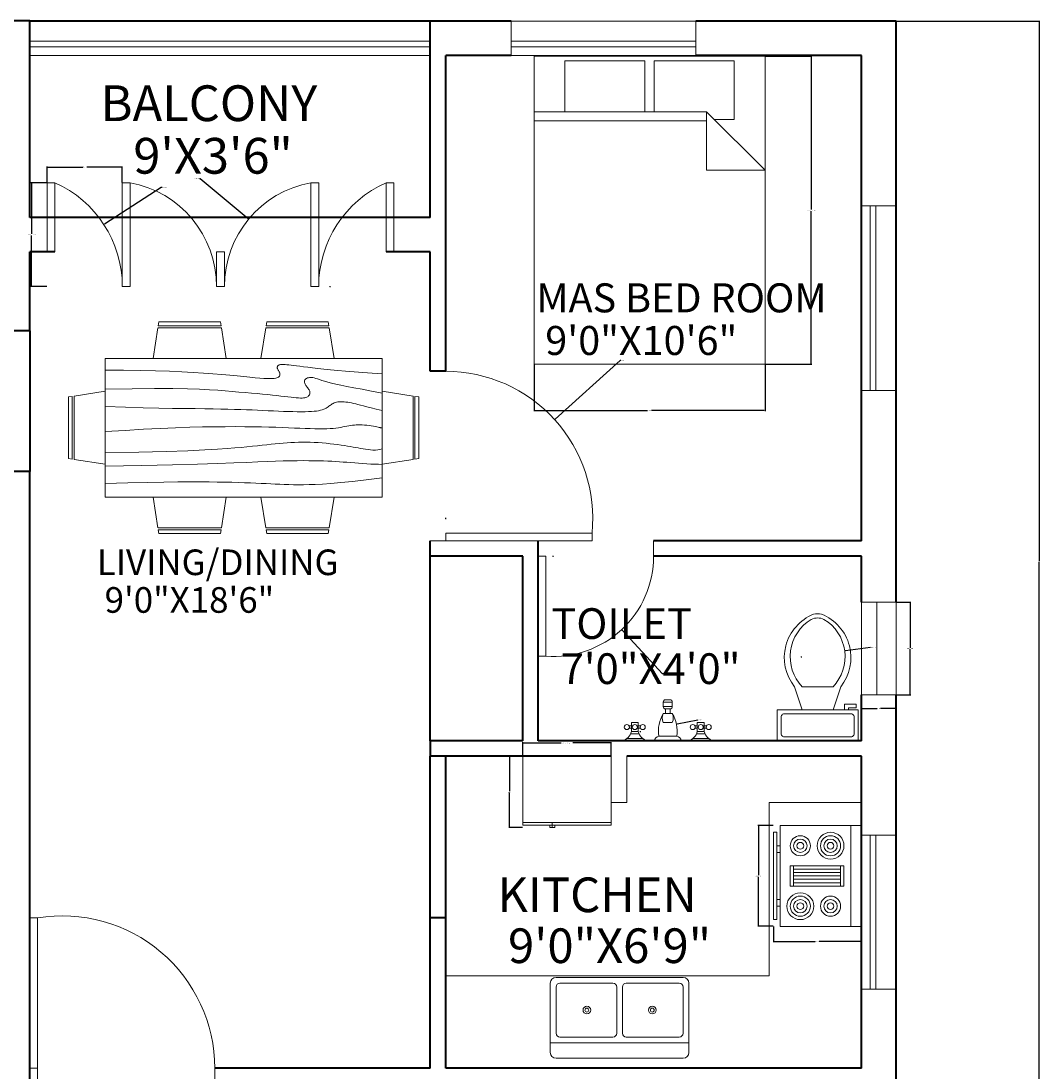
# Model space of a CAD drawing. Units: inches. Extents: x 2220 to 3422, y 783 to 1748.
# Tile 5 of 7: x 2475 to 2740, y 1306 to 1578. Entities that reach past the tile are written whole.
import ezdxf

# ---------------------------------------------------------------- set-up
doc = ezdxf.new("R2010")
doc.units = ezdxf.units.IN
for name, color, linetype, lineweight in [('A-ANNO-DIMS', 2, 'Continuous', 18), ('A-AREA-IDEN', 7, 'Continuous', 18), ('A-DOOR', 3, 'Continuous', 20), ('A-EQPM', 9, 'Continuous', 18), ('A-FLOR-CASE', 8, 'Continuous', 18), ('A-FLOR-FIXT', 9, 'Continuous', 18), ('A-FURN', 8, 'Continuous', 18), ('A-GLAZ', 4, 'Continuous', 18), ('A-WALL', 7, 'Continuous', 40)]:
    doc.layers.add(name, color=color, linetype=linetype, lineweight=lineweight)
doc.styles.get("Standard").update_dxf_attribs({"font": 'arial.ttf'})
doc.dimstyles.get("Standard").update_dxf_attribs({"dimtxt": 0.18, "dimasz": 0.18, "dimexe": 0.18, "dimexo": 0.0625, "dimgap": 0.09, "dimtad": 0, "dimtih": 1, "dimtoh": 1, "dimdec": 4, "dimzin": 0, "dimdsep": 46, "dimtxsty": 'Standard', "dimcen": 0.09, "dimadec": 0, "dimazin": 0, "dimtfac": 1, "dimtdec": 4, "dimtofl": 0, "dimtmove": 0, "dimatfit": 3, "dimfxl": 1, "dimtolj": 1, "dimtzin": 0, "dimarcsym": 0})

# ---------------------------------------------------------------- blocks, each defined once
blk = doc.blocks.new('Range-Oven - 30 in top')
for p, q in [((0, -3), (30, -3)), ((12, -6), (18, -6)), ((13, -20), (13, -6)), ((14, -6), (14, -20)), ((15, -20), (15, -6)), ((16, -6), (16, -20)), ((17, -20), (17, -6)), ((18, -20), (12, -20)), ((6, -24), (6, -25)), ((8, -25), (8, -24)), ((22, -25), (22, -24)), ((24, -24), (24, -25))]:
    blk.add_line(p, q)
for points in [[(0, -24), (0, 0), (30, 0), (30, -24)], [(12, -21), (12, -5), (18, -5), (18, -21)], [(2, -26), (2, -25), (28, -25), (28, -26)]]:
    blk.add_lwpolyline(points, close=True)
for centre, radius in [((6, -9), 4), ((6, -9), 3), ((24, -9), 3), ((6, -9), 2), ((6, -9), 1), ((24, -9), 2), ((24, -9), 1), ((6, -18), 3), ((24, -18), 4), ((24, -18), 3), ((6, -18), 2), ((6, -18), 1), ((24, -18), 2), ((24, -18), 1)]:
    blk.add_circle(centre, radius)
blk = doc.blocks.new('Refrigerator-2 door - 36 in top')
for p, q in [((0, -26.999999), (36, -26.999999)), ((11, -27.999999), (11, -28.999999)), ((11, -28.999999), (13, -28.999999)), ((12, -26.999999), (12, -28.999999)), ((13, -28.999999), (13, -27.999999))]:
    blk.add_line(p, q)
blk.add_lwpolyline([(0, -27.999999), (0, 0), (36, 0), (36, -27.999999)], close=True)
blk = doc.blocks.new('Sink-double - 36 in top')
for p, q in [((-18, -4), (18, -4)), ((-0.75, -18.5), (-0.75, -6.5)), ((0.75, -6.5), (0.75, -18.5))]:
    blk.add_line(p, q)
for points in [[(-16.5, 0), (16.5, 0)], [(-18, -19.5), (-18, -1.5)], [(18, -1.5), (18, -19.5)], [(-16.5, -18.5), (-16.5, -6.5)], [(-15.5, -5.5), (-1.75, -5.5)], [(1.75, -5.5), (15.5, -5.5)], [(16.5, -6.5), (16.5, -18.5)], [(16.5, -21), (-16.5, -21)], [(-1.75, -19.5), (-15.5, -19.5)], [(15.5, -19.5), (1.75, -19.5)]]:
    blk.add_lwpolyline(points)
for centre, radius in [((-8.5, -12.5), 1), ((-8.5, -12.5), 0.5), ((8.5, -12.5), 1), ((8.5, -12.5), 0.5)]:
    blk.add_circle(centre, radius)
for centre, radius, start, end in [((-16.5, -1.5), 1.5, 90, 180), ((16.5, -1.5), 1.5, 0, 90), ((-15.5, -6.5), 1, 90, 180), ((-1.75, -6.5), 1, 0, 90), ((1.75, -6.5), 1, 90, 180), ((15.5, -6.5), 1, 0, 90), ((-15.5, -18.5), 1, 180, 270), ((-1.75, -18.5), 1, 270, 0), ((1.75, -18.5), 1, 180, 270), ((15.5, -18.5), 1, 270, 0), ((-16.5, -19.5), 1.5, 180, 270), ((16.5, -19.5), 1.5, 270, 0)]:
    blk.add_arc(centre, radius, start, end)
blk = doc.blocks.new('Dining Set - 36 x 72 in.')
for p, q in [((-22, 27.5), (-22.1562, 26.50042)), ((-22, 27.5), (-6, 27.5)), ((-5.8437, 26.49966), (-6, 27.5)), ((6, 27.5), (5.8438, 26.50042)), ((6, 27.5), (22, 27.5)), ((22.1563, 26.49966), (22, 27.5)), ((-22.2343, 26.00059), (-23.4847, 17.99762)), ((-22.2304, 26), (-5.7608, 26)), ((-5.8416, 26.5), (-22.1534, 26.5)), ((-4.5152, 17.99762), (-5.7655, 25.99926)), ((5.7657, 26.00059), (4.5153, 17.99762)), ((5.7696, 26), (22.2392, 26)), ((22.1584, 26.5), (5.8466, 26.5)), ((23.4848, 17.99762), (22.2345, 25.99926)), ((36, 18), (-36, 18)), ((-36, 18), (-36, -18)), ((36, -18), (36, 18)), ((-44.0006, 8.23428), (-35.9976, 9.48474)), ((-44, 8.23041), (-44, -8.23915)), ((44.0006, 8.23428), (35.9976, 9.48474)), ((44, 8.23041), (44, -8.23915)), ((-45.5, 8), (-44.5004, 8.15617)), ((-45.5, 8), (-45.5, -8)), ((-44.5, -8.15843), (-44.5, 8.15338)), ((44.5, -8.15843), (44.5, 8.15338)), ((45.5, 8), (44.5005, 8.15617)), ((45.5, 8), (45.5, -8)), ((-44.4997, -8.15631), (-45.5, -8)), ((44.4997, -8.15631), (45.5, -8)), ((-35.9976, -9.48476), (-43.9993, -8.2345)), ((35.9976, -9.48476), (43.9993, -8.2345)), ((-36, -18), (36, -18)), ((-22.2343, -26.0006), (-23.4847, -17.99762)), ((-4.5152, -17.99762), (-5.7655, -25.99928)), ((5.7657, -26.0006), (4.5153, -17.99762)), ((23.4848, -17.99762), (22.2345, -25.99928)), ((-22.2304, -26), (-5.7608, -26)), ((-22, -27.5), (-22.1562, -26.50044)), ((-5.8416, -26.5), (-22.1534, -26.5)), ((-5.8437, -26.49967), (-6, -27.5)), ((5.7696, -26), (22.2392, -26)), ((6, -27.5), (5.8438, -26.50044)), ((22.1584, -26.5), (5.8466, -26.5)), ((22.1563, -26.49967), (22, -27.5)), ((-22, -27.5), (-6, -27.5)), ((6, -27.5), (22, -27.5))]:
    blk.add_line(p, q)
for points in [[(-36, 15), (-31.1772, 14.97754), (-26.8079, 14.91406), (-22.8538, 14.81543), (-19.276, 14.6875), (-16.0362, 14.53613), (-13.0957, 14.36718), (-10.4159, 14.18652), (-7.9583, 14), (-5.6904, 13.81315), (-3.6035, 13.63021), (-1.6954, 13.45508), (0.0365, 13.29166), (1.5945, 13.14388), (2.9811, 13.01562), (4.1988, 12.9108), (5.25, 12.83333), (6.1393, 12.78613), (6.8802, 12.76823), (7.4883, 12.77767), (7.9792, 12.8125), (8.3685, 12.87077), (8.6719, 12.95052), (8.9049, 13.0498), (9.0833, 13.16666), (9.2205, 13.29899), (9.3216, 13.44401), (9.3895, 13.59879), (9.4271, 13.76041), (9.4373, 13.92594), (9.4232, 14.09245), (9.3875, 14.257), (9.3333, 14.41666), (9.2638, 14.56917), (9.1836, 14.71484), (9.0975, 14.85465), (9.0104, 14.98958), (8.9272, 15.1206), (8.8529, 15.2487), (8.7922, 15.37483), (8.75, 15.5), (8.7305, 15.62467), (8.7344, 15.74739), (8.7617, 15.86621), (8.8125, 15.97916), (8.8867, 16.08431), (8.9844, 16.17968), (9.1055, 16.26334), (9.25, 16.33333), (9.4189, 16.38802), (9.6172, 16.42708), (9.8506, 16.45052), (10.125, 16.45833), (10.4463, 16.45052), (10.8203, 16.42708), (11.2529, 16.38802), (11.75, 16.33333), (12.3184, 16.26318), (12.9694, 16.17838), (13.7151, 16.07991), (14.5677, 15.96875), (15.5395, 15.84586), (16.6426, 15.71224), (17.8893, 15.56884), (19.2917, 15.41666), (20.859, 15.25667), (22.5879, 15.08984), (24.4721, 14.91715), (26.5052, 14.73958), (28.6809, 14.5581), (30.9929, 14.3737), (33.4347, 14.18733), (36, 14)], [(-36, 10), (-28.9766, 10.14274), (-23.1725, 10.20442), (-18.4241, 10.19775), (-14.5677, 10.13541), (-11.4399, 10.03011), (-8.877, 9.89453), (-6.7154, 9.74137), (-4.7917, 9.58333), (-2.9698, 9.43082), (-1.2246, 9.28515), (0.4415, 9.14534), (2.026, 9.01041), (3.5266, 8.87939), (4.9408, 8.7513), (6.266, 8.62516), (7.5, 8.5), (8.6411, 8.37549), (9.6914, 8.2539), (10.6538, 8.13818), (11.5312, 8.03125), (12.3267, 7.93603), (13.043, 7.85547), (13.6831, 7.79248), (14.25, 7.75), (14.7471, 7.7303), (15.1797, 7.73307), (15.5537, 7.75732), (15.875, 7.80208), (16.1494, 7.86637), (16.3828, 7.94922), (16.5811, 8.04964), (16.75, 8.16666), (16.8944, 8.29915), (17.0143, 8.44531), (17.1089, 8.60319), (17.1771, 8.77083), (17.218, 8.94629), (17.2305, 9.1276), (17.2137, 9.31282), (17.1667, 9.5), (17.0895, 9.6875), (16.987, 9.875), (16.8649, 10.0625), (16.7292, 10.25), (16.5856, 10.4375), (16.4401, 10.625), (16.2985, 10.8125), (16.1667, 11), (16.05, 11.18733), (15.9518, 11.3737), (15.8752, 11.5581), (15.8229, 11.73958), (15.798, 11.91715), (15.8034, 12.08984), (15.842, 12.25667), (15.9167, 12.41666), (16.0295, 12.56836), (16.1784, 12.70833), (16.3605, 12.83268), (16.5729, 12.9375), (16.8127, 13.01888), (17.0768, 13.07291), (17.3625, 13.0957), (17.6667, 13.08333), (17.9894, 13.03312), (18.3418, 12.94726), (18.7382, 12.82918), (19.1927, 12.68229), (19.7195, 12.51001), (20.3327, 12.31575), (21.0465, 12.10294), (21.875, 11.875), (22.8357, 11.63354), (23.959, 11.37304), (25.2786, 11.08618), (26.8282, 10.76562), (28.6414, 10.40405), (30.752, 9.99414), (33.1936, 9.52856), (36, 9)], [(-36, 5.5), (-30.7157, 5.3348), (-26.069, 5.20963), (-21.9946, 5.11767), (-18.4271, 5.05208), (-15.3009, 5.00602), (-12.5508, 4.97265), (-10.1112, 4.94515), (-7.9167, 4.91666), (-5.909, 4.88167), (-4.0586, 4.83984), (-2.3429, 4.79215), (-0.7396, 4.73958), (0.7739, 4.6831), (2.22, 4.6237), (3.6213, 4.56233), (5, 4.5), (6.373, 4.43782), (7.7344, 4.3776), (9.0723, 4.32129), (10.375, 4.27083), (11.6309, 4.22819), (12.8281, 4.19531), (13.9551, 4.17415), (15, 4.16666), (15.954, 4.17448), (16.819, 4.19791), (17.6001, 4.23698), (18.3021, 4.29166), (18.9299, 4.36198), (19.4883, 4.44791), (19.9823, 4.54948), (20.4167, 4.66666), (20.7969, 4.79899), (21.1302, 4.94401), (21.4245, 5.09879), (21.6875, 5.26041), (21.9271, 5.42594), (22.1511, 5.59245), (22.3672, 5.757), (22.5834, 5.91666), (22.8065, 6.06868), (23.0404, 6.21093), (23.2879, 6.34147), (23.5521, 6.45833), (23.8358, 6.55957), (24.142, 6.64323), (24.4735, 6.70735), (24.8334, 6.75), (25.2235, 6.76969), (25.642, 6.76692), (26.0858, 6.74267), (26.5521, 6.69791), (27.0379, 6.63362), (27.5404, 6.55078), (28.0565, 6.45036), (28.5834, 6.33333), (29.1242, 6.19987), (29.7071, 6.04687), (30.3661, 5.87044), (31.1354, 5.66666), (32.0493, 5.43164), (33.142, 5.16146), (34.4475, 4.85221), (36, 4.5)], [(-36, -1), (-30.7915, -0.6591), (-26.0195, -0.38216), (-21.6519, -0.16284), (-17.6563, 0.00521), (-14.0005, 0.12833), (-10.6523, 0.21289), (-7.5796, 0.26522), (-4.75, 0.29166), (-2.134, 0.29793), (0.2878, 0.28711), (2.5317, 0.26163), (4.6146, 0.22396), (6.5529, 0.17651), (8.3633, 0.12174), (10.0623, 0.06209), (11.6667, 0), (13.1899, -0.06201), (14.6341, -0.1211), (15.9982, -0.17432), (17.2813, -0.21875), (18.4823, -0.25147), (19.6003, -0.26953), (20.6343, -0.27002), (21.5834, -0.25), (22.4481, -0.20768), (23.2357, -0.14584), (23.9549, -0.06836), (24.6146, 0.02083), (25.2235, 0.11784), (25.7904, 0.21875), (26.3241, 0.31966), (26.8334, 0.41666), (27.3265, 0.50618), (27.8099, 0.58593), (28.2894, 0.65397), (28.7709, 0.70833), (29.2601, 0.74707), (29.763, 0.76823), (30.2855, 0.76985), (30.8334, 0.75), (31.4088, 0.70784), (31.9994, 0.64713), (32.589, 0.57275), (33.1615, 0.48958), (33.7008, 0.4025), (34.1908, 0.3164), (34.6153, 0.23616), (34.9584, 0.16666), (35.2099, 0.11165), (35.3848, 0.07031), (35.504, 0.04069), (35.5886, 0.02083), (35.6594, 0.00879), (35.7377, 0.0026), (35.8442, 0.00032), (36, 0)], [(-36, -6.5), (-27.1843, -6.31267), (-20.084, -6.1263), (-14.469, -5.9419), (-10.1094, -5.76042), (-6.7752, -5.58285), (-4.2363, -5.41016), (-2.2629, -5.24333), (-0.625, -5.08334), (0.8708, -4.93099), (2.2715, -4.78646), (3.5872, -4.64974), (4.8281, -4.52084), (6.0046, -4.39974), (7.127, -4.28646), (8.2053, -4.18099), (9.25, -4.08334), (10.2705, -3.99382), (11.2734, -3.91407), (12.2647, -3.84603), (13.25, -3.79167), (14.2354, -3.75293), (15.2266, -3.73177), (16.2295, -3.73015), (17.25, -3.75), (18.2912, -3.79248), (19.3451, -3.85547), (20.4009, -3.93604), (21.4479, -4.03125), (22.4754, -4.13819), (23.4727, -4.25391), (24.4289, -4.37549), (25.3334, -4.5), (26.1785, -4.62492), (26.9694, -4.74935), (27.7145, -4.87281), (28.4219, -4.99479), (29.1, -5.11483), (29.7572, -5.23242), (30.4016, -5.34709), (31.0417, -5.45834), (31.6837, -5.56437), (32.3262, -5.65821), (32.9658, -5.73153), (33.599, -5.77604), (34.2224, -5.78345), (34.8327, -5.74545), (35.4264, -5.65373), (36, -5.5)], [(-36, -10), (-26.4022, -9.81299), (-18.4675, -9.62891), (-11.9839, -9.45069), (-6.7396, -9.28125), (-2.5226, -9.12354), (0.8789, -8.98047), (3.6769, -8.85498), (6.0833, -8.75), (8.2767, -8.66765), (10.3021, -8.60677), (12.1712, -8.56543), (13.8958, -8.54167), (15.4876, -8.53353), (16.9583, -8.53907), (18.3197, -8.55632), (19.5834, -8.58334), (20.7616, -8.61841), (21.8685, -8.66081), (22.9188, -8.71004), (23.9271, -8.76563), (24.9081, -8.82707), (25.8763, -8.89388), (26.8465, -8.96558), (27.8334, -9.04167), (28.8474, -9.12118), (29.8828, -9.20117), (30.93, -9.27824), (31.9792, -9.34896), (33.0205, -9.40991), (34.0443, -9.45768), (35.0407, -9.48885), (36, -9.5)], [(-36, -14.5), (-30.0881, -14.33513), (-25.0332, -14.21224), (-20.7312, -14.12647), (-17.0781, -14.07292), (-13.97, -14.04671), (-11.3027, -14.04297), (-8.9724, -14.05681), (-6.875, -14.08334), (-4.9224, -14.11833), (-3.0905, -14.16016), (-1.3709, -14.20785), (0.2448, -14.26042), (1.7647, -14.3169), (3.1973, -14.3763), (4.5507, -14.43767), (5.8333, -14.5), (7.0554, -14.5621), (8.235, -14.62175), (9.3922, -14.67652), (10.5469, -14.72396), (11.7192, -14.76164), (12.929, -14.78711), (14.1965, -14.79794), (15.5417, -14.79167), (16.9933, -14.76424), (18.6152, -14.70508), (20.4804, -14.60197), (22.6615, -14.44271), (25.2312, -14.21509), (28.2624, -13.9069), (31.8277, -13.50594), (36, -13)]]:
    blk.add_lwpolyline(points)
blk = doc.blocks.new('Toilet - top')
for p, q in [((9.5, -6), (9.5, -2)), ((-8, -8.5), (-8, -8)), ((-7, -8), (-7, -9.5)), ((-4, -8), (-6, -14)), ((4, -8), (6, -14)), ((-10, -8.5), (-8, -8.5)), ((-10, -9.5), (-10, -8.5)), ((-7, -9.5), (-10, -9.5)), ((4, -14), (-4, -14))]:
    blk.add_line(p, q)
blk.add_lwpolyline([(10.5, -8), (10.5, 0), (-10.5, 0), (-10.5, -8)], close=True)
for points in [[(-9.5, -2), (-9.5, -6)], [(8.5, -1), (-8.5, -1)], [(-8.5, -7), (8.5, -7)]]:
    blk.add_lwpolyline(points)
for centre, radius, start, end in [((-8.62, -1.88), 0.884, 81.8699, 188.1301), ((8.62, -1.88), 0.884, 351.8699, 98.1301), ((-8.62, -6.12), 0.884, 171.8699, 278.1301), ((8.62, -6.12), 0.884, 261.8699, 8.1301), ((3.52, -21.58), 12.17, 141.4691, 247.9714), ((4.2, -21.82), 11.33, 136.3677, 238.9468), ((-3.52, -21.58), 12.17, 292.0284, 38.5307), ((-4.2, -21.82), 11.33, 301.053, 43.6321), ((0, -27.88), 4, 245.7318, 294.2682), ((0, -29), 4, 254.8605, 285.1395)]:
    blk.add_arc(centre, radius, start, end)
blk = doc.blocks.new('Faucet - Bathroom front')
for p, q in [((-0.5, 4.25), (0.5, 4.25)), ((0.5, 3.75), (-0.5, 3.75)), ((-0.25, 3), (-0.25, 3.5)), ((0.25, 3.5), (0.25, 3)), ((-0.5, 3), (0.5, 3)), ((-4, 1.625), (-4.25, 1.625)), ((-4, 1.375), (-4.25, 1.375)), ((-3.25, 1.625), (-3, 1.625)), ((-3.25, 1.375), (-3, 1.375)), ((0.5, 2), (-0.5, 2)), ((3.25, 1.625), (3, 1.625)), ((3.25, 1.375), (3, 1.375)), ((4, 1.625), (4.25, 1.625)), ((4, 1.375), (4.25, 1.375)), ((-5, 0), (-2.25, 0)), ((-4.5087, 0.25), (-2.7408, 0.25)), ((-3.1442, 0.75), (-4.0979, 0.75)), ((-1.5, 0), (1.5, 0)), ((-1, 0.5), (1, 0.5)), ((2.25, 0), (5, 0)), ((2.7413, 0.25), (4.5092, 0.25)), ((4.1058, 0.75), (3.1521, 0.75))]:
    blk.add_line(p, q)
for points in [[(-0.5, 3.75), (-0.5, 4.25)], [(-0.25, 4.5), (0.25, 4.5)], [(0.25, 3.5), (-0.25, 3.5)], [(0.5, 4.25), (0.5, 3.75)]]:
    blk.add_lwpolyline(points)
for points in [[(-4, 1), (-4, 2), (-3.25, 2), (-3.25, 1)], [(3.25, 1), (3.25, 2), (4, 2), (4, 1)]]:
    blk.add_lwpolyline(points, close=True)
for centre in [(-4.5, 1.5), (-3.625, 1.5), (-2.75, 1.5), (2.75, 1.5), (3.625, 1.5), (4.5, 1.5)]:
    blk.add_circle(centre, 0.2795)
for centre, radius, start, end in [((-0.2575, 4.2575), 0.2426, 88.22243, 181.7776), ((-0.2575, 3.7425), 0.2426, 178.2224, 271.7776), ((0.2575, 4.2575), 0.2426, 358.2224, 91.77757), ((0.2575, 3.7425), 0.2426, 268.2224, 1.777565), ((3, 1), 4.0311, 150.2551, 187.125), ((0.6413, 2.5), 1.246, 156.3417, 203.6583), ((-3, 1), 4.0311, 352.875, 29.74488), ((-0.6413, 2.5), 1.246, 336.3417, 23.65835), ((-5.375, 1.375), 1.4252, 285.2551, 344.7449), ((-1.875, 1.375), 1.4252, 195.2551, 254.7449), ((-0.7962, -0.2038), 0.7327, 106.1502, 163.8498), ((0.7962, -0.2038), 0.7327, 16.1502, 73.84979), ((1.875, 1.375), 1.4252, 285.2551, 344.7449), ((5.375, 1.375), 1.4252, 195.2551, 254.7449)]:
    blk.add_arc(centre, radius, start, end)
blk = doc.blocks.new('Bed - Queen')
for p, q in [((0, -80.00003), (0, 0)), ((0, 0), (59.99999, 0)), ((59.99999, 0), (59.99999, -80.00003)), ((7.99999, -1.2), (28.79998, -1.2)), ((7.99999, -14.4), (7.99999, -1.2)), ((28.79998, -1.2), (28.79998, -14.4)), ((31.19999, -1.2), (51.99999, -1.2)), ((31.19999, -14.4), (31.19999, -1.2)), ((51.99999, -1.2), (51.99999, -16.4)), ((0, -14.4), (44.8, -14.4)), ((59.99999, -29.6), (44.8, -14.4)), ((44.8, -14.4), (44.8, -29.6)), ((44.8, -16.8), (0, -16.8)), ((51.99999, -16.4), (46.79936, -16.4)), ((44.8, -29.6), (59.99999, -29.6)), ((59.99999, -80.00003), (0, -80.00003))]:
    blk.add_line(p, q)
blk = doc.blocks.new('DOOR-UNIT-ENTRY')
for p, q in [((0, 48.53), (2, 48.53)), ((2, 0.53), (2, 48.53)), ((48, 39.53), (48, 48.53)), ((0, 39.53), (2, 39.53)), ((0, 0.53), (2, 0.53))]:
    blk.add_line(p, q)
blk.add_arc((8.47, 39.53), 39.53, 260.5843, 0)
blk = doc.blocks.new('DOOR-BATH-SWING')
for p, q in [((30, 26.06), (30, 30.06)), ((0, 26.06), (2, 26.06)), ((2, 0.06), (2, 26.06)), ((0, 0.06), (2, 0.06))]:
    blk.add_line(p, q)
blk.add_arc((3.93, 26.06), 26.07, 265.7578, 0)
blk = doc.blocks.new('DOOR-BALCONY-CENTER')
for p, q in [((0, 0), (0, 27)), ((0, 27), (2, 27)), ((2, 0), (2, 27)), ((24.5, 27), (24.5, 18)), ((24.5, 27), (26.5, 27)), ((26.5, 27), (26.5, 18)), ((49, 27), (49, 0)), ((49, 27), (51, 27)), ((51, 27), (51, 0)), ((0, 0), (2, 0)), ((49, 0), (51, 0))]:
    blk.add_line(p, q)
for centre, start, end in [((-2.95, 27), 280.3889, 0), ((53.95, 27), 180, 259.6111)]:
    blk.add_arc(centre, 27.45, start, end)
blk = doc.blocks.new('DOOR-BALCONY-END-B')
for p, q in [((0, 27), (0, 9)), ((0, 27), (2, 27)), ((2, 27), (2, 9))]:
    blk.add_line(p, q)
blk.add_arc((-10.08, 0), 29.58, 0, 65.8984)
blk = doc.blocks.new('WIN-48-OFFSET-A')
for p, q in [((0, 0), (0, 9)), ((0, 9), (48, 9)), ((48, 0), (48, 9)), ((0, 6.75), (48, 6.75)), ((0, 5.25), (48, 5.25)), ((0, 0), (48, 0))]:
    blk.add_line(p, q)
blk = doc.blocks.new('VENT-24-SINGLE')
for p, q in [((0, 24), (9, 24)), ((0, 24), (0, 0)), ((4, 0), (4, 24)), ((9, 24), (9, 0)), ((0, 0), (9, 0))]:
    blk.add_line(p, q)
blk = doc.blocks.new('*D19')
at = {"layer": 'A-ANNO-DIMS', "color": 0, "lineweight": -2, "transparency": 16777216}
for p, q in [((2668.55, 1569.22), (2680.66, 1569.22)), ((2680.48, 1569.04), (2680.48, 1529.41)), ((2680.48, 1489.4), (2680.48, 1529.03)), ((2668.55, 1489.22), (2680.66, 1489.22))]:
    blk.add_line(p, q, dxfattribs=at)
at = {"layer": 'A-ANNO-DIMS', "color": 0, "transparency": 16777216}
for points in [[(2680.45, 1569.04), (2680.51, 1569.04), (2680.48, 1569.22)], [(2680.45, 1489.4), (2680.51, 1489.4), (2680.48, 1489.22)]]:
    blk.add_solid(points, dxfattribs=at)
at = {"layer": 'Defpoints', "color": 0, "transparency": 16777216}
for p in [(2668.48, 1569.22), (2680.48, 1569.22), (2668.48, 1489.22)]:
    blk.add_point(p, dxfattribs=at)
at = {"layer": 'A-ANNO-DIMS', "color": 0, "transparency": 16777216, "insert": (2680.48, 1529.22), "char_height": 0.18, "attachment_point": 5}
blk.add_mtext('\\A1;QUEEN BED 80 TYP.', dxfattribs=at)
blk = doc.blocks.new('*D20')
at = {"layer": 'A-ANNO-DIMS', "color": 0, "lineweight": -2, "transparency": 16777216}
for p, q in [((2608.48, 1489.16), (2608.48, 1477.04)), ((2668.48, 1489.16), (2668.48, 1477.04)), ((2608.66, 1477.22), (2637.95, 1477.22)), ((2668.3, 1477.22), (2639.01, 1477.22))]:
    blk.add_line(p, q, dxfattribs=at)
at = {"layer": 'A-ANNO-DIMS', "color": 0, "transparency": 16777216}
for points in [[(2608.66, 1477.25), (2608.66, 1477.19), (2608.48, 1477.22)], [(2668.3, 1477.25), (2668.3, 1477.19), (2668.48, 1477.22)]]:
    blk.add_solid(points, dxfattribs=at)
at = {"layer": 'Defpoints', "color": 0, "transparency": 16777216}
for p in [(2608.48, 1489.22), (2668.48, 1489.22), (2668.48, 1477.22)]:
    blk.add_point(p, dxfattribs=at)
at = {"layer": 'A-ANNO-DIMS', "color": 0, "transparency": 16777216, "insert": (2638.48, 1477.22), "char_height": 0.18, "attachment_point": 5}
blk.add_mtext('\\A1;60 TYP.', dxfattribs=at)
blk = doc.blocks.new('*D27')
at = {"layer": 'A-ANNO-DIMS', "color": 0, "lineweight": -2, "transparency": 16777216}
for p, q in [((2670.61, 1369.38), (2666.57, 1369.38)), ((2666.75, 1369.2), (2666.75, 1356.48)), ((2666.75, 1343.4), (2666.75, 1356.12)), ((2670.61, 1343.22), (2666.57, 1343.22))]:
    blk.add_line(p, q, dxfattribs=at)
at = {"layer": 'A-ANNO-DIMS', "color": 0, "transparency": 16777216}
for points in [[(2666.72, 1369.2), (2666.78, 1369.2), (2666.75, 1369.38)], [(2666.72, 1343.4), (2666.78, 1343.4), (2666.75, 1343.22)]]:
    blk.add_solid(points, dxfattribs=at)
at = {"layer": 'Defpoints', "color": 0, "transparency": 16777216}
for p in [(2670.68, 1369.38), (2666.75, 1343.22), (2670.68, 1343.22)]:
    blk.add_point(p, dxfattribs=at)
at = {"layer": 'A-ANNO-DIMS', "color": 0, "transparency": 16777216, "insert": (2666.75, 1356.3), "char_height": 0.18, "attachment_point": 5}
blk.add_mtext('\\A1;RANGE 26 TYP.', dxfattribs=at)
blk = doc.blocks.new('*D28')
at = {"layer": 'A-ANNO-DIMS', "color": 0, "lineweight": -2, "transparency": 16777216}
for p, q in [((2670.68, 1343.16), (2670.68, 1339.11)), ((2693.35, 1343.16), (2693.35, 1339.11)), ((2670.86, 1339.29), (2681.48, 1339.29)), ((2693.17, 1339.29), (2682.54, 1339.29))]:
    blk.add_line(p, q, dxfattribs=at)
at = {"layer": 'A-ANNO-DIMS', "color": 0, "transparency": 16777216}
for points in [[(2670.86, 1339.32), (2670.86, 1339.26), (2670.68, 1339.29)], [(2693.17, 1339.32), (2693.17, 1339.26), (2693.35, 1339.29)]]:
    blk.add_solid(points, dxfattribs=at)
at = {"layer": 'Defpoints', "color": 0, "transparency": 16777216}
for p in [(2670.68, 1343.22), (2693.35, 1343.22), (2693.35, 1339.29)]:
    blk.add_point(p, dxfattribs=at)
at = {"layer": 'A-ANNO-DIMS', "color": 0, "transparency": 16777216, "insert": (2682.01, 1339.29), "char_height": 0.18, "attachment_point": 5}
blk.add_mtext('\\A1;23 TYP.', dxfattribs=at)
blk = doc.blocks.new('*D37')
at = {"layer": 'A-ANNO-DIMS', "color": 0, "lineweight": -2, "transparency": 16777216}
for p, q in [((2605.54, 1387.48), (2605.54, 1391.05)), ((2628.55, 1387.48), (2628.55, 1391.05)), ((2605.72, 1390.87), (2615.49, 1390.87)), ((2628.37, 1390.87), (2618.6, 1390.87))]:
    blk.add_line(p, q, dxfattribs=at)
at = {"layer": 'A-ANNO-DIMS', "color": 0, "transparency": 16777216}
for points in [[(2605.72, 1390.9), (2605.72, 1390.84), (2605.54, 1390.87)], [(2628.37, 1390.9), (2628.37, 1390.84), (2628.55, 1390.87)]]:
    blk.add_solid(points, dxfattribs=at)
at = {"layer": 'Defpoints', "color": 0, "transparency": 16777216}
for p in [(2628.55, 1390.87), (2605.54, 1387.41), (2628.55, 1387.41)]:
    blk.add_point(p, dxfattribs=at)
at = {"layer": 'A-ANNO-DIMS', "color": 0, "transparency": 16777216, "insert": (2617.04, 1390.87), "char_height": 0.18, "attachment_point": 5}
blk.add_mtext('\\A1;REFRIGERATOR 23 TYP.', dxfattribs=at)
blk = doc.blocks.new('*D38')
at = {"layer": 'A-ANNO-DIMS', "color": 0, "lineweight": -2, "transparency": 16777216}
for p, q in [((2605.48, 1387.41), (2601.91, 1387.41)), ((2602.09, 1387.23), (2602.09, 1378.33)), ((2602.09, 1369.06), (2602.09, 1377.97)), ((2605.48, 1368.88), (2601.91, 1368.88))]:
    blk.add_line(p, q, dxfattribs=at)
at = {"layer": 'A-ANNO-DIMS', "color": 0, "transparency": 16777216}
for points in [[(2602.06, 1387.23), (2602.12, 1387.23), (2602.09, 1387.41)], [(2602.06, 1369.06), (2602.12, 1369.06), (2602.09, 1368.88)]]:
    blk.add_solid(points, dxfattribs=at)
at = {"layer": 'Defpoints', "color": 0, "transparency": 16777216}
for p in [(2602.09, 1387.41), (2605.54, 1387.41), (2605.54, 1368.88)]:
    blk.add_point(p, dxfattribs=at)
at = {"layer": 'A-ANNO-DIMS', "color": 0, "transparency": 16777216, "insert": (2602.09, 1378.15), "char_height": 0.18, "attachment_point": 5}
blk.add_mtext('\\A1;19 TYP.', dxfattribs=at)
blk = doc.blocks.new('*D47')
at = {"layer": 'A-ANNO-DIMS', "color": 0, "lineweight": -2, "transparency": 16777216}
for p, q in [((2481.98, 1536.39), (2477.82, 1536.39)), ((2478, 1536.21), (2478, 1523.07)), ((2478, 1509.57), (2478, 1522.71)), ((2481.98, 1509.39), (2477.82, 1509.39))]:
    blk.add_line(p, q, dxfattribs=at)
at = {"layer": 'A-ANNO-DIMS', "color": 0, "transparency": 16777216}
for points in [[(2477.97, 1536.21), (2478.03, 1536.21), (2478, 1536.39)], [(2477.97, 1509.57), (2478.03, 1509.57), (2478, 1509.39)]]:
    blk.add_solid(points, dxfattribs=at)
at = {"layer": 'Defpoints', "color": 0, "transparency": 16777216}
for p in [(2478, 1536.39), (2482.05, 1536.39), (2482.05, 1509.39)]:
    blk.add_point(p, dxfattribs=at)
at = {"layer": 'A-ANNO-DIMS', "color": 0, "transparency": 16777216, "insert": (2478, 1522.89), "char_height": 0.18, "attachment_point": 5}
blk.add_mtext('\\A1;END LEAF B 27 TYP.', dxfattribs=at)
blk = doc.blocks.new('*D48')
at = {"layer": 'A-ANNO-DIMS', "color": 0, "lineweight": -2, "transparency": 16777216}
for p, q in [((2482.05, 1536.45), (2482.05, 1540.62)), ((2482.23, 1540.44), (2491.27, 1540.44)), ((2501.37, 1540.44), (2492.33, 1540.44)), ((2501.55, 1536.45), (2501.55, 1540.62))]:
    blk.add_line(p, q, dxfattribs=at)
at = {"layer": 'A-ANNO-DIMS', "color": 0, "transparency": 16777216}
for points in [[(2482.23, 1540.47), (2482.23, 1540.41), (2482.05, 1540.44)], [(2501.37, 1540.47), (2501.37, 1540.41), (2501.55, 1540.44)]]:
    blk.add_solid(points, dxfattribs=at)
at = {"layer": 'Defpoints', "color": 0, "transparency": 16777216}
for p in [(2501.55, 1540.44), (2482.05, 1536.39), (2501.55, 1536.39)]:
    blk.add_point(p, dxfattribs=at)
at = {"layer": 'A-ANNO-DIMS', "color": 0, "transparency": 16777216, "insert": (2491.8, 1540.44), "char_height": 0.18, "attachment_point": 5}
blk.add_mtext('\\A1;20 TYP.', dxfattribs=at)
blk = doc.blocks.new('*D51')
at = {"layer": 'A-ANNO-DIMS', "color": 0, "lineweight": -2, "transparency": 16777216}
for p, q in [((2702.61, 1427.39), (2706.33, 1427.39)), ((2706.15, 1427.21), (2706.15, 1415.57)), ((2706.15, 1403.57), (2706.15, 1415.21)), ((2702.61, 1403.39), (2706.33, 1403.39))]:
    blk.add_line(p, q, dxfattribs=at)
at = {"layer": 'A-ANNO-DIMS', "color": 0, "transparency": 16777216}
for points in [[(2706.12, 1427.21), (2706.18, 1427.21), (2706.15, 1427.39)], [(2706.12, 1403.57), (2706.18, 1403.57), (2706.15, 1403.39)]]:
    blk.add_solid(points, dxfattribs=at)
at = {"layer": 'Defpoints', "color": 0, "transparency": 16777216}
for p in [(2702.55, 1427.39), (2706.15, 1427.39), (2702.55, 1403.39)]:
    blk.add_point(p, dxfattribs=at)
at = {"layer": 'A-ANNO-DIMS', "color": 0, "transparency": 16777216, "insert": (2706.15, 1415.39), "char_height": 0.18, "attachment_point": 5}
blk.add_mtext('\\A1;VENT 24 TYP.', dxfattribs=at)
blk = doc.blocks.new('*D52')
at = {"layer": 'A-ANNO-DIMS', "color": 0, "lineweight": -2, "transparency": 16777216}
for p, q in [((2693.55, 1403.33), (2693.55, 1399.61)), ((2702.55, 1403.33), (2702.55, 1399.61)), ((2693.73, 1399.79), (2697.59, 1399.79)), ((2702.37, 1399.79), (2698.5, 1399.79))]:
    blk.add_line(p, q, dxfattribs=at)
at = {"layer": 'A-ANNO-DIMS', "color": 0, "transparency": 16777216}
for points in [[(2693.73, 1399.82), (2693.73, 1399.76), (2693.55, 1399.79)], [(2702.37, 1399.82), (2702.37, 1399.76), (2702.55, 1399.79)]]:
    blk.add_solid(points, dxfattribs=at)
at = {"layer": 'Defpoints', "color": 0, "transparency": 16777216}
for p in [(2693.55, 1403.39), (2702.55, 1403.39), (2702.55, 1399.79)]:
    blk.add_point(p, dxfattribs=at)
at = {"layer": 'A-ANNO-DIMS', "color": 0, "transparency": 16777216, "insert": (2698.05, 1399.79), "char_height": 0.18, "attachment_point": 5}
blk.add_mtext('\\A1;9 TYP.', dxfattribs=at)
blk = doc.blocks.new('*D56')
at = {"layer": 'A-ANNO-DIMS', "color": 0, "lineweight": -2, "transparency": 16777216}
for p, q in [((2702.61, 1578.39), (2739.88, 1578.39)), ((2739.7, 1578.21), (2739.7, 1438.07)), ((2739.7, 1297.57), (2739.7, 1437.71)), ((2702.61, 1297.39), (2739.88, 1297.39))]:
    blk.add_line(p, q, dxfattribs=at)
at = {"layer": 'A-ANNO-DIMS', "color": 0, "transparency": 16777216}
for points in [[(2739.67, 1578.21), (2739.73, 1578.21), (2739.7, 1578.39)], [(2739.67, 1297.57), (2739.73, 1297.57), (2739.7, 1297.39)]]:
    blk.add_solid(points, dxfattribs=at)
at = {"layer": 'Defpoints', "color": 0, "transparency": 16777216}
for p in [(2702.55, 1578.39), (2739.7, 1578.39), (2702.55, 1297.39)]:
    blk.add_point(p, dxfattribs=at)
at = {"layer": 'A-ANNO-DIMS', "color": 0, "transparency": 16777216, "insert": (2739.7, 1437.89), "char_height": 0.18, "attachment_point": 5}
blk.add_mtext('\\A1;281', dxfattribs=at)
blk = doc.blocks.new('*D77')
at = {"layer": 'A-ANNO-DIMS', "color": 0, "lineweight": -2, "transparency": 16777216}
for p, q in [((2630.86, 1490.2), (2614, 1474.94)), ((2631.04, 1490.2), (2630.86, 1490.2)), ((2585.46, 1449.2), (2585.64, 1449.2)), ((2585.55, 1449.11), (2585.55, 1449.29))]:
    blk.add_line(p, q, dxfattribs=at)
at = {"layer": 'A-ANNO-DIMS', "color": 0, "transparency": 16777216}
blk.add_solid([(2613.98, 1474.97), (2614.02, 1474.92), (2613.87, 1474.82)], dxfattribs=at)
at = {"layer": 'Defpoints', "color": 0, "transparency": 16777216}
for p in [(2613.87, 1474.82), (2585.55, 1449.2)]:
    blk.add_point(p, dxfattribs=at)
at = {"layer": 'A-ANNO-DIMS', "color": 0, "transparency": 16777216, "insert": (2631.52, 1490.2), "char_height": 0.18, "attachment_point": 5}
blk.add_mtext('\\A1;R38.19', dxfattribs=at)
blk = doc.blocks.new('*D82')
at = {"layer": 'A-ANNO-DIMS', "color": 0, "lineweight": -2, "transparency": 16777216}
for p, q in [((2511.68, 1535.13), (2496.94, 1525.58)), ((2511.86, 1535.13), (2511.68, 1535.13)), ((2471.88, 1509.39), (2472.06, 1509.39)), ((2471.97, 1509.3), (2471.97, 1509.48))]:
    blk.add_line(p, q, dxfattribs=at)
at = {"layer": 'A-ANNO-DIMS', "color": 0, "transparency": 16777216}
blk.add_solid([(2496.92, 1525.6), (2496.96, 1525.55), (2496.79, 1525.48)], dxfattribs=at)
at = {"layer": 'Defpoints', "color": 0, "transparency": 16777216}
for p in [(2496.79, 1525.48), (2471.97, 1509.39)]:
    blk.add_point(p, dxfattribs=at)
at = {"layer": 'A-ANNO-DIMS', "color": 0, "transparency": 16777216, "insert": (2512.54, 1535.13), "char_height": 0.18, "attachment_point": 5}
blk.add_mtext('\\A1;2X R29.58', dxfattribs=at)
blk = doc.blocks.new('*D83')
at = {"layer": 'A-ANNO-DIMS', "color": 0, "lineweight": -2, "transparency": 16777216}
for p, q in [((2521.58, 1537.51), (2521.76, 1537.51)), ((2521.76, 1537.51), (2534.27, 1527.08)), ((2555.41, 1509.39), (2555.59, 1509.39)), ((2555.5, 1509.3), (2555.5, 1509.48))]:
    blk.add_line(p, q, dxfattribs=at)
at = {"layer": 'A-ANNO-DIMS', "color": 0, "transparency": 16777216}
blk.add_solid([(2534.29, 1527.1), (2534.25, 1527.06), (2534.41, 1526.96)], dxfattribs=at)
at = {"layer": 'Defpoints', "color": 0, "transparency": 16777216}
for p in [(2534.41, 1526.96), (2555.5, 1509.39)]:
    blk.add_point(p, dxfattribs=at)
at = {"layer": 'A-ANNO-DIMS', "color": 0, "transparency": 16777216, "insert": (2520.9, 1537.51), "char_height": 0.18, "attachment_point": 5}
blk.add_mtext('\\A1;4X R27.45', dxfattribs=at)
blk = doc.blocks.new('*D84')
at = {"layer": 'A-ANNO-DIMS', "color": 0, "lineweight": -2, "transparency": 16777216}
for p, q in [((2613.39, 1439.39), (2613.57, 1439.39)), ((2613.48, 1439.3), (2613.48, 1439.48)), ((2641.86, 1408.82), (2631.34, 1420.15)), ((2642.04, 1408.82), (2641.86, 1408.82))]:
    blk.add_line(p, q, dxfattribs=at)
at = {"layer": 'A-ANNO-DIMS', "color": 0, "transparency": 16777216}
blk.add_solid([(2631.36, 1420.17), (2631.32, 1420.13), (2631.22, 1420.29)], dxfattribs=at)
at = {"layer": 'Defpoints', "color": 0, "transparency": 16777216}
for p in [(2613.48, 1439.39), (2631.22, 1420.29)]:
    blk.add_point(p, dxfattribs=at)
at = {"layer": 'A-ANNO-DIMS', "color": 0, "transparency": 16777216, "insert": (2642.71, 1408.82), "char_height": 0.18, "attachment_point": 5}
blk.add_mtext('\\A1;3X R26.07', dxfattribs=at)
blk = doc.blocks.new('*D89')
at = {"layer": 'A-ANNO-DIMS', "color": 0, "lineweight": -2, "transparency": 16777216}
for p, q in [((2695.91, 1415.67), (2689.35, 1414.79)), ((2677.85, 1413.25), (2678.03, 1413.25)), ((2677.94, 1413.16), (2677.94, 1413.34))]:
    blk.add_line(p, q, dxfattribs=at)
at = {"layer": 'A-ANNO-DIMS', "color": 0, "transparency": 16777216}
blk.add_solid([(2689.35, 1414.82), (2689.35, 1414.76), (2689.17, 1414.76)], dxfattribs=at)
at = {"layer": 'Defpoints', "color": 0, "transparency": 16777216}
for p in [(2677.94, 1413.25), (2689.17, 1414.76)]:
    blk.add_point(p, dxfattribs=at)
at = {"layer": 'A-ANNO-DIMS', "color": 0, "transparency": 16777216, "insert": (2696.58, 1415.67), "char_height": 0.18, "attachment_point": 5}
blk.add_mtext('\\A1;8X R11.33', dxfattribs=at)
blk = doc.blocks.new('*D90')
at = {"layer": 'A-ANNO-DIMS', "color": 0, "lineweight": -2, "transparency": 16777216}
for p, q in [((2651.07, 1396.79), (2645.65, 1395.7)), ((2636.05, 1393.8), (2636.23, 1393.8)), ((2636.14, 1393.71), (2636.14, 1393.89))]:
    blk.add_line(p, q, dxfattribs=at)
at = {"layer": 'A-ANNO-DIMS', "color": 0, "transparency": 16777216}
blk.add_solid([(2645.64, 1395.73), (2645.66, 1395.67), (2645.47, 1395.67)], dxfattribs=at)
at = {"layer": 'Defpoints', "color": 0, "transparency": 16777216}
for p in [(2636.14, 1393.8), (2645.47, 1395.67)]:
    blk.add_point(p, dxfattribs=at)
at = {"layer": 'A-ANNO-DIMS', "color": 0, "transparency": 16777216, "insert": (2651.68, 1396.79), "char_height": 0.18, "attachment_point": 5}
blk.add_mtext('\\A1;8X R9.52', dxfattribs=at)

msp = doc.modelspace()

# ---------------------------------------------------------------- linework, layer by layer
at = {"layer": 'A-DOOR'}
for p, q in [((2526.0466, 1518.3907), (2528.0466, 1518.3907)), ((2623.5466, 1443.3907), (2581.5466, 1443.3907)), ((2585.5466, 1443.3907), (2585.5466, 1445.3907)), ((2623.5466, 1445.3907), (2585.5466, 1445.3907)), ((2623.5466, 1443.3907), (2623.5466, 1445.3907)), ((2479.5466, 1306.3907), (2477.5466, 1306.3907))]:
    msp.add_line(p, q, dxfattribs=at)
msp.add_arc((2585.5466, 1449.2002), 38.1905, 354.27519, 90, dxfattribs=at)
at = {"layer": 'A-FLOR-CASE'}
for p, q in [((2628.5471, 1387.3907), (2628.5471, 1375.3907)), ((2632.5471, 1387.3907), (2632.5471, 1375.3907)), ((2632.5471, 1375.3907), (2628.5471, 1375.3907)), ((2669.5466, 1330.3907), (2669.5466, 1375.3907)), ((2693.5466, 1375.3907), (2669.5466, 1375.3907)), ((2669.5466, 1330.3907), (2585.5466, 1330.3907))]:
    msp.add_line(p, q, dxfattribs=at)
at = {"layer": 'A-GLAZ'}
for p, q in [((2581.5466, 1573.1407), (2477.5466, 1573.1407)), ((2581.5466, 1571.6407), (2477.5466, 1571.6407)), ((2581.5466, 1569.3907), (2477.5466, 1569.3907)), ((2702.5466, 1366.8907), (2693.5466, 1366.8907)), ((2695.7966, 1326.8907), (2695.7966, 1366.8907)), ((2697.2966, 1326.8907), (2697.2966, 1366.8907)), ((2702.5466, 1326.8907), (2693.5466, 1326.8907))]:
    msp.add_line(p, q, dxfattribs=at)
at = {"layer": 'A-WALL'}
for p, q in [((2477.5466, 1578.3907), (2409.5466, 1578.3907)), ((2477.5466, 1578.3907), (2602.5466, 1578.3907)), ((2477.5466, 1527.3907), (2477.5466, 1578.3907)), ((2581.5466, 1527.3907), (2581.5466, 1578.3907)), ((2581.5466, 1527.3907), (2581.5466, 1578.3907)), ((2650.5466, 1578.3907), (2702.5466, 1578.3907)), ((2702.5466, 1530.3907), (2702.5466, 1578.3907)), ((2585.5466, 1487.3907), (2585.5466, 1569.3907)), ((2602.5466, 1569.3907), (2585.5466, 1569.3907)), ((2693.5466, 1569.3907), (2650.5466, 1569.3907)), ((2693.5466, 1530.3907), (2693.5466, 1569.3907)), ((2693.5466, 1443.3907), (2693.5466, 1530.3907)), ((2702.5466, 1427.3907), (2702.5466, 1530.3907)), ((2581.5466, 1527.3907), (2477.5466, 1527.3907)), ((2477.5466, 1497.8907), (2477.5466, 1518.3907)), ((2484.0466, 1518.3907), (2477.5466, 1518.3907)), ((2581.5466, 1518.3907), (2570.0466, 1518.3907)), ((2581.5466, 1487.3907), (2581.5466, 1518.3907)), ((2581.5466, 1497.8907), (2581.5466, 1518.3907)), ((2477.5466, 1497.8907), (2471.5466, 1497.8907)), ((2477.5466, 1497.8907), (2477.5466, 1461.3907)), ((2585.5466, 1487.3907), (2581.5466, 1487.3907)), ((2477.5466, 1461.3907), (2413.5466, 1461.3907)), ((2477.5466, 1109.8907), (2477.5466, 1461.3907)), ((2581.5466, 1391.3907), (2581.5466, 1443.3907)), ((2609.5466, 1391.3907), (2609.5466, 1443.3907)), ((2693.5466, 1443.3907), (2639.5466, 1443.3907)), ((2605.5466, 1439.3907), (2581.5466, 1439.3907)), ((2605.5466, 1391.3907), (2605.5466, 1439.3907)), ((2693.5466, 1439.3907), (2639.5466, 1439.3907)), ((2693.5466, 1427.3907), (2693.5466, 1439.3907)), ((2693.5466, 1391.3907), (2693.5466, 1403.3907)), ((2702.5466, 1297.3907), (2702.5466, 1403.3907)), ((2581.5466, 1391.3907), (2581.5466, 1387.3907)), ((2605.5466, 1391.3907), (2581.5466, 1391.3907)), ((2693.5466, 1391.3907), (2609.5466, 1391.3907)), ((2581.5466, 1345.3907), (2581.5466, 1387.3907)), ((2628.5471, 1387.3907), (2581.5466, 1387.3907)), ((2585.5466, 1345.3907), (2585.5466, 1387.3907)), ((2693.5466, 1387.3907), (2632.5471, 1387.3907)), ((2693.5466, 1306.3907), (2693.5466, 1387.3907)), ((2581.5466, 1306.3907), (2581.5466, 1345.3907)), ((2585.5466, 1345.3907), (2581.5466, 1345.3907)), ((2585.5466, 1306.3907), (2585.5466, 1345.3907)), ((2581.5466, 1306.3907), (2525.5466, 1306.3907)), ((2693.5466, 1306.3907), (2585.5466, 1306.3907))]:
    msp.add_line(p, q, dxfattribs=at)

# ---------------------------------------------------------------- block references
at = {"layer": 'A-DOOR'}
for name, p in [('DOOR-BALCONY-END-B', (2482.047, 1509.391)), ('DOOR-BATH-SWING', (2609.547, 1413.326))]:
    msp.add_blockref(name, p, dxfattribs=at)
at = {"layer": 'A-DOOR', "rotation": 180}
msp.add_blockref('DOOR-BALCONY-CENTER', (2552.5463, 1536.3904), dxfattribs=at)
at = {"layer": 'A-DOOR', "extrusion": (0, 0, -1), "zscale": -1}
msp.add_blockref('DOOR-BALCONY-END-B', (-2572.0463, 1509.391), dxfattribs=at)
at = {"layer": 'A-DOOR', "extrusion": (0, 0, -1), "zscale": -1, "rotation": 180}
msp.add_blockref('DOOR-UNIT-ENTRY', (-2477.547, 1345.9234), dxfattribs=at)
at = {"layer": 'A-EQPM', "xscale": 0.6390408655968428, "yscale": 0.6390408655968428, "zscale": 0.6390408655968428}
msp.add_blockref('Refrigerator-2 door - 36 in top', (2605.5416, 1387.4145), dxfattribs=at)
at = {"layer": 'A-EQPM', "xscale": 0.8722005701805317, "yscale": 0.8722005701805317, "zscale": 0.8722005701805317, "rotation": 270}
msp.add_blockref('Range-Oven - 30 in top', (2693.3531, 1369.3837), dxfattribs=at)
at = {"layer": 'A-FLOR-FIXT', "rotation": 180}
msp.add_blockref('Toilet - top', (2682.1427, 1391.4374), dxfattribs=at)
at = {"layer": 'A-FLOR-FIXT', "xscale": 2.361580970438625, "yscale": 2.361580970438625, "zscale": 2.361580970438625}
msp.add_blockref('Faucet - Bathroom front', (2643.2231, 1391.4374), dxfattribs=at)
at = {"layer": 'A-FLOR-FIXT', "xscale": -1, "rotation": 180}
msp.add_blockref('Sink-double - 36 in top', (2630.7033, 1308.9605), dxfattribs=at)
at = {"layer": 'A-FURN'}
for name, p in [('Bed - Queen', (2608.4834, 1569.22)), ('Dining Set - 36 x 72 in.', (2533.0492, 1472.7204))]:
    msp.add_blockref(name, p, dxfattribs=at)
at = {"layer": 'A-GLAZ'}
for p, rotation in [((2650.5463, 1578.3904), 180), ((2702.5463, 1482.3911), 89.99999999999532)]:
    msp.add_blockref('WIN-48-OFFSET-A', p, dxfattribs=dict(at, rotation=rotation))
msp.add_blockref('VENT-24-SINGLE', (2693.547, 1403.391), dxfattribs=at)

# ---------------------------------------------------------------- texts
at = {"layer": 'A-AREA-IDEN'}
for s, height, p in [('BALCONY', 9.29088, (2495.8793, 1552.3846)), ('   9\'X3\'6"', 9.29088, (2495.8793, 1538.7301)), ('MAS BED ROOM', 7.536224, (2609.0967, 1502.7099)), (' 9\'0"X10\'6"', 7.536224, (2609.0967, 1491.6341)), ('LIVING/DINING', 6.656123, (2494.9116, 1434.4539)), (' 9\'0"X18\'6"', 6.656123, (2494.9116, 1424.6716)), ('TOILET', 7.97038, (2612.9538, 1417.8805)), (' 7\'0"X4\'0"', 7.97038, (2612.9538, 1406.1666)), ('KITCHEN', 9, (2598.9711, 1346.9073)), (' 9\'0"X6\'9"', 9, (2598.9711, 1333.6803))]:
    msp.add_text(s, height=height, dxfattribs=at).set_placement(p)

# ---------------------------------------------------------------- dimensions: what is measured, and where the dimension line sits
at = {"layer": 'A-ANNO-DIMS'}
dim = msp.add_linear_dim(base=(2739.6966, 1578.3907), p1=(2702.5466, 1297.3907), p2=(2702.5466, 1578.3907), angle=90, dimstyle='Standard', override={"dimdec": 0, "dimlfac": 1, "dimrnd": 0, "dimzin": 0, "dimdsep": 46, "dimlunit": 2}, dxfattribs=at)
dim.commit()
dim.dimension.update_dxf_attribs({"geometry": '*D56', "text_midpoint": (2739.6966, 1437.8907)})
for base, p1, p2, angle, text, picture, middle in [((2680.4834, 1569.22), (2668.4834, 1489.2199), (2668.4834, 1569.22), 90, 'QUEEN BED <> TYP.', '*D19', (2680.4834, 1529.2199)), ((2477.9966, 1536.3907), (2482.0466, 1509.3907), (2482.0466, 1536.3907), 90, 'END LEAF B <> TYP.', '*D47', (2477.9966, 1522.8907)), ((2706.1466, 1427.3907), (2702.5466, 1403.3907), (2702.5466, 1427.3907), 90, 'VENT <> TYP.', '*D51', (2706.1466, 1415.3907)), ((2602.0908, 1387.4145), (2605.5416, 1368.8823), (2605.5416, 1387.4145), 90, '<> TYP.', '*D38', (2602.0908, 1378.1484)), ((2666.751, 1343.2177), (2670.6759, 1369.3837), (2670.6759, 1343.2177), 270, 'RANGE <> TYP.', '*D27', (2666.751, 1356.3007))]:
    dim = msp.add_linear_dim(base=base, p1=p1, p2=p2, angle=angle, text=text, dimstyle='Standard', override={"dimdec": 0, "dimlfac": 1, "dimrnd": 0, "dimzin": 0, "dimdsep": 46, "dimlunit": 2}, dxfattribs=at)
    dim.commit()
    dim.dimension.update_dxf_attribs({"geometry": picture, "text_midpoint": middle})
for base, p1, p2, text, picture, middle in [((2501.5466333189, 1540.4406899565), (2482.0466333189, 1536.3906899565), (2501.5466333189, 1536.3906899565), '<> TYP.', '*D48', (2491.7966333189, 1540.4406899565)), ((2668.4834, 1477.2199), (2608.4834, 1489.2199), (2668.4834, 1489.2199), '<> TYP.', '*D20', (2638.4834, 1477.2199)), ((2702.5466, 1399.7907), (2693.5466, 1403.3907), (2702.5466, 1403.3907), '<> TYP.', '*D52', (2698.0466, 1399.7907)), ((2628.5471, 1390.8653), (2605.5416, 1387.4145), (2628.5471, 1387.4145), 'REFRIGERATOR <> TYP.', '*D37', (2617.0443, 1390.8653)), ((2693.3531, 1339.2928), (2670.6759, 1343.2177), (2693.3531, 1343.2177), '<> TYP.', '*D28', (2682.0145, 1339.2928))]:
    dim = msp.add_linear_dim(base=base, p1=p1, p2=p2, text=text, dimstyle='Standard', override={"dimdec": 0, "dimlfac": 1, "dimrnd": 0, "dimzin": 0, "dimdsep": 46, "dimlunit": 2}, dxfattribs=at)
    dim.commit()
    dim.dimension.update_dxf_attribs({"geometry": picture, "text_midpoint": middle})
for center, mpoint, text, picture, middle in [((2555.4966, 1509.3907), (2534.4091, 1526.9639), '4X <>', '*D83', (2520.8991, 1537.5079)), ((2471.9681, 1509.3907), (2496.7892, 1525.4781), '2X <>', '*D82', (2512.5368, 1535.1306)), ((2613.4752, 1439.3907), (2631.2159, 1420.2861), '3X <>', '*D84', (2642.7135, 1408.8233)), ((2677.9427, 1413.2548), (2689.171, 1414.764), '8X <>', '*D89', (2695.9079, 1415.6695)), ((2636.1383, 1393.799), (2645.4733, 1395.6661), '8X <>', '*D90', (2651.0743, 1396.7863))]:
    dim = msp.add_radius_dim(center=center, mpoint=mpoint, text=text, dimstyle='Standard', override={"dimdec": 2, "dimlfac": 1, "dimrnd": 0, "dimzin": 0, "dimdsep": 46, "dimlunit": 2}, dxfattribs=at)
    dim.commit()
    dim.dimension.update_dxf_attribs({"geometry": picture, "text_midpoint": middle, "dimtype": 164})
dim = msp.add_radius_dim(center=(2585.5466, 1449.2002), mpoint=(2613.866, 1474.823), dimstyle='Standard', override={"dimdec": 2, "dimlfac": 1, "dimrnd": 0, "dimzin": 0, "dimdsep": 46, "dimlunit": 2}, dxfattribs=at)
dim.commit()
dim.dimension.update_dxf_attribs({"geometry": '*D77', "text_midpoint": (2631.5176, 1490.1967), "dimtype": 164})

doc.saveas('drawing.dxf')
